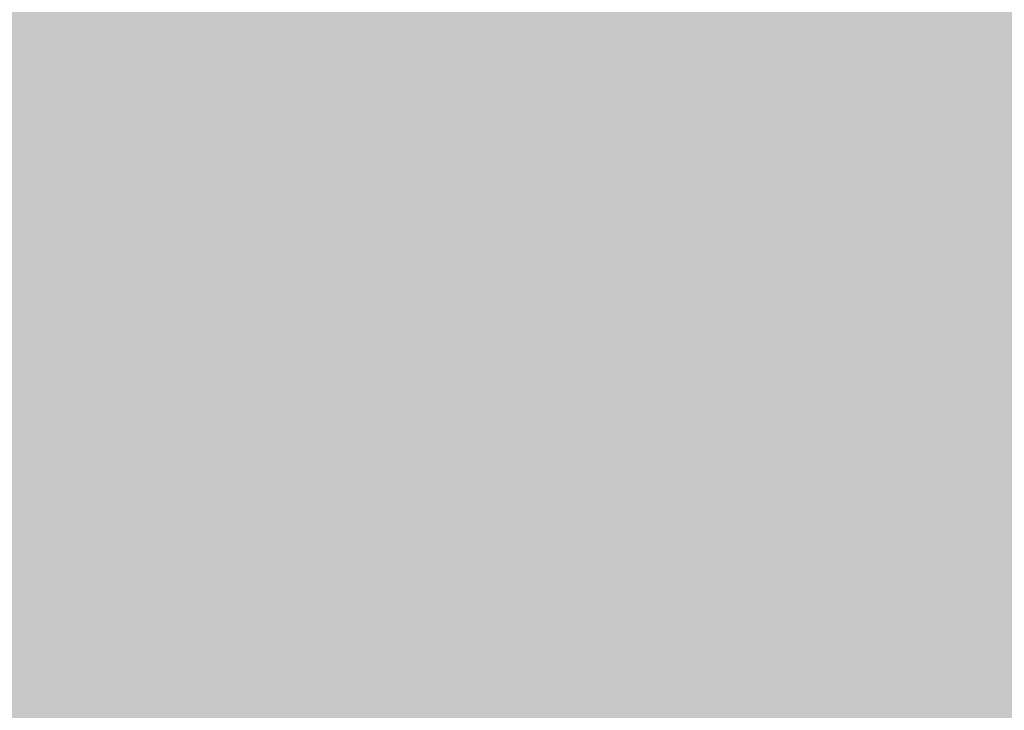
# Model space of a CAD drawing. Units: inches. Extents: x 2091 to 2899, y 967 to 2217.
# Tile 165 of 256: x 2203.144443 to 2203.14684, y 1152.248741 to 1152.250422. Entities that reach past the tile are written whole.
import ezdxf

# ---------------------------------------------------------------- set-up
doc = ezdxf.new("R2010")
doc.units = ezdxf.units.IN
doc.layers.add('A-WALL-PATT', color=141, linetype='Continuous', lineweight=13, true_color=0xadddf7)

msp = doc.modelspace()

# ---------------------------------------------------------------- hatches: boundary and pattern name
at = {"layer": 'A-WALL-PATT'}
h = msp.add_hatch(color=256, dxfattribs=at)
h.dxf.hatch_style = 1
h.paths.add_polyline_path([(2803.1436027, 2050.9190588), (2203.1436027, 2050.9190588), (2203.1436027, 1090.9190588), (2803.1436027, 1090.9190588)])
h.paths.add_polyline_path([(2635.7988501, 1147.5404649), (2674.5240524, 1147.5404649, 0.376086), (2678.5296653, 1152.8802017), (2678.5296653, 1159.5564734, 0.333335), (2674.524319, 1163.561846), (2674.524319, 1163.5618504), (2674.524319, 1192.9343904), (2635.8059707, 1192.9343904), (2597.0876225, 1192.9343904), (2597.0876225, 1163.561846, 0.333335), (2593.0822761, 1159.5564734), (2593.0822761, 1152.8802017, 0.376086), (2597.087889, 1147.5404649)], flags=0)
h.paths.add_polyline_path([(2436.0104329, 1278.2407784, 0.000483), (2435.9526433, 1278.215027, -0.001328), (2435.9356253, 1278.1116934, -0.001711), (2436.1164401, 1278.0407583, 0.002185)], flags=0)
h.paths.add_polyline_path([(2794.1436027, 1143.4190588), (2794.1436027, 1347.4190588), (2543.3701706, 1347.4190588), (2543.3701706, 1351.9190588), (2794.1436027, 1351.9190588), (2794.1436027, 1392.7135549), (2793.9473982, 1392.7135549), (2793.9473982, 1473.5368999), (2794.1436027, 1473.5368999), (2794.1436027, 1531.9190588), (2650.1436027, 1531.9190588), (2650.1436027, 1536.4190588), (2794.1436027, 1536.4190588), (2794.1436027, 1692.4190588), (2609.3756095, 1692.4190588), (2609.3756095, 1644.4190588), (2604.8756095, 1644.4190588), (2604.8756095, 1744.9190588), (2609.3756095, 1744.9190588), (2609.3756095, 1696.9190588), (2794.1436027, 1696.9190588), (2794.1436027, 1780.9190588), (2609.6436027, 1780.9190588), (2493.8756095, 1780.9190588), (2493.8756095, 1785.4190588), (2609.6436027, 1785.4190588), (2794.1436027, 1785.4190588), (2794.1436027, 1847.9388214), (2793.9512217, 1847.9388214), (2793.9512217, 1928.7621663), (2794.1436027, 1928.7621663), (2794.1436027, 1941.4190588), (2614.1436027, 1941.4190588), (2614.1436027, 1821.4190588), (2609.6436027, 1821.4190588), (2609.6436027, 1941.4190588), (2392.1436027, 1941.4190588), (2392.1436027, 1819.9190588), (2387.6436027, 1819.9190588), (2387.6436027, 1941.4190588), (2212.1436027, 1941.4190588), (2212.1436027, 1783.9190588), (2392.1436027, 1783.9190588), (2392.1436027, 1780.9190588), (2212.1436027, 1780.9190588), (2212.1436027, 1629.4190588), (2387.6436027, 1629.4190588), (2387.6436027, 1744.9190588), (2392.1436027, 1744.9190588), (2392.1436027, 1627.9190588), (2317.1436027, 1627.9190588), (2317.1436027, 1551.4190588), (2317.1436027, 1536.4190588), (2459.3835909, 1536.4190588), (2459.3835909, 1602.3964802), (2463.8835909, 1602.3964802), (2463.8835909, 1531.9190588), (2456.6436027, 1531.9190588), (2456.6436027, 1529.9190588), (2452.1436027, 1529.9190588), (2452.1436027, 1531.9190588), (2312.6436027, 1531.9190588), (2312.6436027, 1551.4190588), (2306.1436027, 1551.4190588), (2306.1436027, 1555.9190588), (2308.1436027, 1555.9190588), (2308.1436027, 1551.4190588), (2312.6436027, 1551.4190588), (2312.6436027, 1627.9190588), (2212.1436027, 1627.9190588), (2212.1436027, 1555.9190588), (2270.1436027, 1555.9190588), (2270.1436027, 1551.4190588), (2212.1436027, 1551.4190588), (2212.1436027, 1351.9190588), (2272.1436027, 1351.9190588), (2272.1436027, 1347.4190588), (2212.1436027, 1347.4190588), (2212.1436027, 1275.4190588), (2308.1436027, 1275.4190588), (2308.1436027, 1351.9190588), (2452.1436027, 1351.9190588), (2452.1436027, 1493.9190588), (2456.6436027, 1493.9190588), (2456.6436027, 1347.4190588), (2312.6436027, 1347.4190588), (2312.6436027, 1270.9190588), (2212.1436027, 1270.9190588), (2212.1436027, 1099.9190588), (2281.2375229, 1099.9190588), (2282.8710413, 1110.9138034), (2282.0083413, 1116.9966034), (2278.5577413, 1121.4204034), (2268.2056413, 1128.0562034), (2272.0876413, 1128.0562034), (2273.8129413, 1131.9270034), (2279.4203413, 1134.6919034), (2285.0278413, 1135.2449034), (2287.6158413, 1137.4568034), (2288.0471413, 1138.0098034), (2289.3411413, 1140.7747034), (2291.0665413, 1139.6687034), (2292.3605413, 1135.2449034), (2295.3798413, 1136.9038034), (2296.2425413, 1135.7979034), (2297.1052413, 1133.0330034), (2300.1246413, 1138.0098034), (2303.1439413, 1138.0098034), (2304.4379413, 1135.7979034), (2303.1439413, 1133.5860034), (2306.5946413, 1134.6919034), (2307.8887413, 1133.0330034), (2310.9080413, 1135.2449034), (2313.9274413, 1134.1389034), (2315.6268599, 1132.4271023), (2308.3200413, 1117.5496034), (2290.2038413, 1109.8079034), (2288.9098413, 1103.1721034), (2289.2723086, 1099.9190588), (2434.9182274, 1099.9190588), (2431.5932274, 1124.7880588), (2429.9302274, 1169.5530588), (2430.9271848, 1240.5196942), (2435.6589255, 1238.1861258), (2437.1352274, 1196.5540588), (2438.7982274, 1143.9730588), (2442.6782274, 1111.9980588), (2446.5582274, 1099.9190588), (2794.1436027, 1099.9190588), (2794.1436027, 1138.9190588), (2548.0324471, 1138.9190588), (2548.0324471, 1143.4190588), (2548.0324471, 1148.8190588), (2546.6684571, 1148.0315588), (2528.6856919, 1179.1786218, 0.256256), (2512.0324471, 1148.8190588), (2512.0324471, 1143.4190588), (2512.0324471, 1138.9190588), (2507.5324471, 1138.9190588), (2507.5324471, 1143.4190588), (2507.5324471, 1148.8190588, 0.256256), (2490.8792023, 1179.1786218), (2472.8964371, 1148.0315588), (2471.5324471, 1148.8190588), (2471.5324471, 1143.4190588), (2467.0324471, 1143.4190588), (2467.0324471, 1269.9457858, 0.039061), (2460.9099871, 1273.5800588), (2467.0324471, 1273.5800588), (2467.0324471, 1286.3253638, 0.014511), (2465.2161944, 1286.7619052), (2467.0324471, 1287.0525761), (2467.0324471, 1323.4190588), (2471.5324471, 1323.4190588), (2471.5324471, 1148.8190588), (2489.5324471, 1179.9959734), (2490.8964371, 1179.2084734), (2490.8792023, 1179.1786218, -0.256256), (2507.5324471, 1148.8190588), (2507.5324471, 1143.4190588), (2512.0324471, 1143.4190588), (2512.0324471, 1148.8190588, -0.256256), (2528.6856919, 1179.1786218), (2528.6684571, 1179.2084734), (2530.0324471, 1179.9959734), (2548.0324471, 1148.8190588), (2548.0324471, 1143.4190588)], flags=16)
h.paths.add_polyline_path([(2607.7685461, 1200.9450832), (2607.7685461, 1265.0306251), (2597.0876225, 1281.0520106), (2619.7845852, 1281.0520106), (2627.795278, 1337.1268598), (2635.7988501, 1337.1268598), (2643.8166634, 1337.1268598), (2651.8273562, 1281.0520106), (2674.524319, 1281.0520106), (2663.8433953, 1265.0306251), (2663.8433953, 1200.9450832), (2635.8059707, 1200.9450832)], flags=0)
edge = h.paths.add_edge_path(flags=0)
edge.add_ellipse((13303.8962153, 1272.9987247), major_axis=(-10595.3130399, 0.0000005), ratio=0.842303870086, start_angle=0.62823721906, end_angle=0.64655409989, ccw=False)
edge.add_ellipse((2711.7004495, 1156.8526781), major_axis=(2.2197691, 0), ratio=0.84230387, start_angle=111.5352435, end_angle=180.6282372, ccw=False)
edge.add_ellipse((13303.1562922, 1272.9987246), major_axis=(-10593.0263064, 0), ratio=0.842303869544, start_angle=0.52827147182, end_angle=0.64655409706, ccw=False)
edge.add_line((2710.7645961, 1175.3332951), (2710.1299858, 1175.3332951))
edge.add_ellipse((2710.1299858, 1176.5797752), major_axis=(1.4798461, 0), ratio=0.84230387, start_angle=180, end_angle=270, ccw=False)
edge.add_line((2708.6501397, 1176.5797752), (2708.6501397, 1200.7829144))
edge.add_ellipse((2710.1299858, 1200.7829144), major_axis=(1.4798461, 0), ratio=0.84230387, start_angle=90, end_angle=180, ccw=False)
edge.add_line((2710.1299858, 1202.0293944), (2710.4650752, 1202.0293944))
edge.add_ellipse((13303.1562922, 1272.9987246), major_axis=(-10593.0263064, 0), ratio=0.842303869544, start_angle=-0.09022908859, end_angle=0.38386677879, ccw=False)
edge.add_ellipse((2710.1299858, 1290.9270308), major_axis=(-1.4798461, 0), ratio=0.84230387, start_angle=0, end_angle=90, ccw=False)
edge.add_line((2708.6501397, 1290.9270308), (2708.6501397, 1315.13017))
edge.add_ellipse((2710.1299858, 1315.13017), major_axis=(-1.4798461, 0), ratio=0.84230387, start_angle=-90, end_angle=0, ccw=False)
edge.add_line((2710.1299858, 1316.3766501), (2710.7063141, 1316.3766501))
edge.add_ellipse((3238.4017202, 1296.2895655), major_axis=(528.2339998, 0), ratio=0.84230386954, start_angle=176.349572414, end_angle=177.820049686, ccw=False)
edge.add_ellipse((2775.0630432, 1071.4506962), major_axis=(313.3077613, 0), ratio=0.84230386954, start_angle=102.125965552, end_angle=103.780528989, ccw=False)
edge.add_ellipse((2775.0630432, 1078.3056979), major_axis=(-305.3028915, 0), ratio=0.84230386955, start_angle=-79.790461003, end_angle=-77.555372706, ccw=False)
edge.add_ellipse((2695.1417666, 1541.9753825), major_axis=(-250.9602162, 0), ratio=0.84230386954, start_angle=99.256566007, end_angle=102.554932644)
edge.add_line((2741.4103262, 1334.2142554), (2747.1325454, 1337.3784768))
edge.add_ellipse((2747.5386163, 1336.8574776), major_axis=(-0.739923, 0), ratio=0.84230387, start_angle=270, end_angle=307.9331305, ccw=False)
edge.add_ellipse((2747.5386163, 1336.8574776), major_axis=(-0.739923, 0), ratio=0.84230387, start_angle=232.0668695, end_angle=270, ccw=False)
edge.add_line((2747.9446872, 1337.3784768), (2753.6669064, 1334.2142554))
edge.add_ellipse((2799.935466, 1541.9753825), major_axis=(250.9602162, 0), ratio=0.84230386954, start_angle=257.445067356, end_angle=260.743433993)
edge.add_ellipse((2720.0141894, 1078.3056979), major_axis=(305.3028915, 0), ratio=0.84230386954, start_angle=77.555372707, end_angle=79.790461003, ccw=False)
edge.add_ellipse((2720.0141894, 1071.4506962), major_axis=(-313.3077613, 0), ratio=0.84230386954, start_angle=256.219471011, end_angle=257.874034448, ccw=False)
edge.add_ellipse((2256.6755124, 1296.2895655), major_axis=(-528.2339998, 0), ratio=0.84230386954, start_angle=182.179950314, end_angle=183.650427586, ccw=False)
edge.add_line((2784.3709184, 1316.3766501), (2784.9472468, 1316.3766501))
edge.add_ellipse((2784.9472468, 1315.13017), major_axis=(1.4798461, 0), ratio=0.84230387, start_angle=0, end_angle=90, ccw=False)
edge.add_line((2786.4270928, 1315.13017), (2786.4270928, 1290.9270308))
edge.add_ellipse((2784.9472468, 1290.9270308), major_axis=(1.4798461, 0), ratio=0.84230387, start_angle=270, end_angle=360, ccw=False)
edge.add_ellipse((-7808.0790596, 1272.9987246), major_axis=(10593.0263063, 0), ratio=0.842303869544, start_angle=-0.38386677879, end_angle=0.09022908859, ccw=False)
edge.add_line((2784.6121574, 1202.0293944), (2784.9472468, 1202.0293944))
edge.add_ellipse((2784.9472468, 1200.7829144), major_axis=(1.4798461, 0), ratio=0.84230387, start_angle=0, end_angle=90, ccw=False)
edge.add_line((2786.4270928, 1200.7829144), (2786.4270928, 1176.5797752))
edge.add_ellipse((2784.9472468, 1176.5797752), major_axis=(-1.4798461, 0), ratio=0.84230387, start_angle=90, end_angle=180, ccw=False)
edge.add_line((2784.9472468, 1175.3332951), (2784.3126365, 1175.3332951))
edge.add_ellipse((-7808.0790596, 1272.9987246), major_axis=(10593.0263063, 0), ratio=0.842303869544, start_angle=-0.61864319632, end_angle=-0.52827147182, ccw=False)
edge.add_ellipse((2783.3767831, 1156.8526781), major_axis=(-2.2197691, 0), ratio=0.84230387, start_angle=179.3717628, end_angle=248.4647566, ccw=False)
edge.add_ellipse((-7808.8189826, 1272.9987246), major_axis=(-10595.3130398, 0.0000036), ratio=0.842303865762, start_angle=179.3534459226, end_angle=179.37176280343, ccw=False)
edge.add_ellipse((2780.2973026, 1153.500793), major_axis=(-5.2464256, 0), ratio=0.84230387, start_angle=90, end_angle=179.3534459, ccw=False)
edge.add_line((2780.2973026, 1149.0817084), (2714.77993, 1149.0817084))
edge.add_ellipse((2714.77993, 1153.500793), major_axis=(5.2464256, 0), ratio=0.84230387, start_angle=180.6465541, end_angle=270, ccw=False)
edge = h.paths.add_edge_path(flags=0)
edge.add_line((2718.1873674, 1151.0078329), (2718.1873674, 1170.4723638))
edge.add_ellipse((2721.1470595, 1170.4723638), major_axis=(-2.9596921, 0), ratio=0.84230387, start_angle=-90, end_angle=0, ccw=False)
edge.add_line((2721.1470595, 1172.965324), (2773.9301731, 1172.965324))
edge.add_ellipse((2773.9301731, 1170.4723638), major_axis=(-2.9596921, 0), ratio=0.84230387, start_angle=180, end_angle=270, ccw=False)
edge.add_line((2776.8898652, 1170.4723638), (2776.8898652, 1151.0078329))
edge.add_line((2776.8898652, 1151.0078329), (2718.1873674, 1151.0078329))
edge = h.paths.add_edge_path(flags=0)
edge.add_line((2718.1873674, 1180.2341502), (2718.1873674, 1199.0578342))
edge.add_ellipse((2747.5386163, 1320.3986402), major_axis=(147.0179239, 0), ratio=0.84230386954, start_angle=256.40186531, end_angle=283.59813469)
edge.add_line((2776.8898652, 1199.0578342), (2776.8898652, 1180.2341502))
edge.add_ellipse((2747.5386163, 1301.5749562), major_axis=(147.0179239, 0), ratio=0.84230386954, start_angle=256.40186531, end_angle=283.59813469, ccw=False)
edge = h.paths.add_edge_path(flags=0)
edge.add_ellipse((13303.1562922, 1272.9987246), major_axis=(-10591.5464603, 0), ratio=0.842303869555, start_angle=0.05559431352, end_angle=0.37776419393, ccw=False)
edge.add_line((2711.6168595, 1262.7217103), (2715.6674076, 1249.4953957))
edge.add_ellipse((6413.8919626, 1241.691919), major_axis=(-3698.2361592, 0), ratio=0.842303869547, start_angle=-0.120897369, end_angle=0.3640763489)
edge.add_line((2715.7610383, 1218.1924547), (2711.9343065, 1203.167361))
edge = h.paths.add_edge_path(flags=0)
edge.add_line((2718.1873674, 1251.074566), (2716.0024854, 1267.4504351))
edge.add_ellipse((2742.1511746, 1202.1895399), major_axis=(81.7725845, 0), ratio=0.8423038695, start_angle=94.277420963, end_angle=111.834953797, ccw=False)
edge.add_line((2737.0097482, 1270.9306255), (2758.0674844, 1270.9306255))
edge.add_ellipse((2752.926058, 1202.1895399), major_axis=(81.7725845, 0), ratio=0.8423038695, start_angle=68.165046203, end_angle=85.722579037, ccw=False)
edge.add_line((2779.0747472, 1267.4504351), (2776.8898652, 1251.074566))
edge.add_ellipse((2750.3380588, 1187.8853558), major_axis=(79.5796641, 0), ratio=0.8423038695, start_angle=67.208085122, end_angle=85.129930403)
edge.add_line((2756.0346562, 1254.7436557), (2739.0425764, 1254.7436557))
edge.add_ellipse((2744.7391738, 1187.8853558), major_axis=(79.5796641, 0), ratio=0.8423038695, start_angle=94.870069597, end_angle=112.791914878)
edge = h.paths.add_edge_path(flags=0)
edge.add_line((2783.1429261, 1203.167361), (2779.3161943, 1218.1924547))
edge.add_ellipse((-918.81473, 1241.691919), major_axis=(3698.2361592, 0), ratio=0.842303869546, start_angle=-0.3640763489, end_angle=0.120897369)
edge.add_line((2779.409825, 1249.4953957), (2783.4603731, 1262.7217103))
edge.add_ellipse((-7808.0790596, 1272.9987246), major_axis=(-10591.5464603, 0), ratio=0.84230386954, start_angle=179.6222358061, end_angle=179.94440568651, ccw=False)
edge = h.paths.add_edge_path(flags=0)
edge.add_ellipse((2734.2008921, 1286.6904402), major_axis=(-0.3566086, 6.3400775), ratio=0.603833576, start_angle=89.00201428, end_angle=253.65740805, ccw=False)
edge.add_line((2730.3690013, 1286.5418057), (2730.3690013, 1301.3519803))
edge.add_line((2730.3690013, 1301.3519803), (2735.9133107, 1305.2148028))
edge.add_ellipse((2736.3849168, 1304.7345612), major_axis=(0.739923, 0), ratio=0.84230387, start_angle=90, end_angle=134.4802109, ccw=False)
edge.add_line((2736.3849168, 1305.3578013), (2738.0327829, 1305.3578013))
edge.add_line((2738.0327829, 1305.3578013), (2738.0327829, 1307.7079274))
edge.add_ellipse((2794.201642, 1307.7079274), major_axis=(56.168859, 0), ratio=0.8423038695, start_angle=150.5614304, end_angle=180, ccw=False)
edge.add_ellipse((2700.8755906, 1307.7079274), major_axis=(-56.168859, 0), ratio=0.8423038695, start_angle=180, end_angle=209.4385696, ccw=False)
edge.add_line((2757.0444497, 1307.7079274), (2757.0444497, 1305.3578013))
edge.add_line((2757.0444497, 1305.3578013), (2758.6923157, 1305.3578013))
edge.add_ellipse((2758.6923157, 1304.7345612), major_axis=(-0.739923, 0), ratio=0.84230387, start_angle=225.5197891, end_angle=270, ccw=False)
edge.add_line((2759.1639219, 1305.2148028), (2764.7082312, 1301.3519803))
edge.add_line((2764.7082312, 1301.3519803), (2764.7082312, 1286.5418057))
edge.add_ellipse((2760.8763405, 1286.6904402), major_axis=(0.3566086, 6.3400775), ratio=0.603833576, start_angle=106.34259195, end_angle=270.99798572, ccw=False)
edge.add_line((2757.0444497, 1285.7970896), (2757.0444497, 1307.7079274))
edge.add_ellipse((2700.8755906, 1307.7079274), major_axis=(-56.168859, 0), ratio=0.8423038695, start_angle=180, end_angle=209.4385696)
edge.add_ellipse((2794.201642, 1307.7079274), major_axis=(56.168859, 0), ratio=0.8423038695, start_angle=150.5614304, end_angle=180)
edge.add_line((2738.0327829, 1307.7079274), (2738.0327829, 1285.7970896))
h.paths.add_polyline_path([(2417.8122727, 1104.449704), (2413.4922727, 1102.529704), (2410.6122727, 1103.969704), (2409.1722727, 1106.369704), (2407.2522727, 1107.329704), (2406.2922727, 1109.729704), (2405.3322727, 1114.049704), (2405.3322727, 1117.889704), (2406.2922727, 1120.129704), (2407.2522727, 1119.809704), (2408.8483218, 1118.3276585), (2410.1739451, 1119.4241703), (2410.2112727, 1120.405704), (2411.0407305, 1121.4190541), (2410.6992727, 1119.858704), (2410.1739451, 1119.4241703), (2410.0884515, 1117.1761095), (2411.1328361, 1116.2063237), (2413.9722727, 1119.329704), (2416.8522727, 1120.769704), (2416.8697209, 1120.7987842), (2417.0350713, 1119.4051162), (2417.8962134, 1118.1433844), (2418.2922727, 1118.369704), (2419.5444467, 1120.0392692), (2419.3609153, 1118.387487), (2419.0321078, 1119.3561507), (2418.3989394, 1118.5119262), (2419.2522727, 1114.529704), (2418.7940909, 1107.1987949)], flags=0)
h.paths.add_polyline_path([(2508.8701706, 1347.4190588), (2508.3701706, 1347.4190588), (2508.3701706, 1351.9190588), (2508.8701706, 1351.9190588)], flags=0)
h.paths.add_polyline_path([(2473.3701706, 1347.4190588), (2472.3701706, 1347.4190588), (2467.8701706, 1347.4190588), (2467.8701706, 1455.4190588), (2472.3701706, 1455.4190588), (2472.3701706, 1352.4190588), (2473.3701706, 1352.4190588)], flags=0)
h.paths.add_polyline_path([(2352.106244, 1217.4461971), (2349.226244, 1218.8861971), (2347.786244, 1221.2861971), (2345.866244, 1222.2461971), (2344.906244, 1224.6461971), (2343.946244, 1228.9661971), (2343.946244, 1232.8061971), (2344.906244, 1235.0461971), (2345.866244, 1234.7261971), (2347.4622931, 1233.2441515), (2348.7879164, 1234.3406634), (2348.825244, 1235.3221971), (2349.6547018, 1236.3355471), (2349.313244, 1234.7751971), (2348.7879164, 1234.3406634), (2348.7024228, 1232.0926025), (2349.7468074, 1231.1228168), (2352.586244, 1234.2461971), (2355.466244, 1235.6861971), (2355.4836921, 1235.7152773), (2355.6490426, 1234.3216093), (2356.5101846, 1233.0598774), (2356.906244, 1233.2861971), (2358.1584179, 1234.9557623), (2357.9748866, 1233.3039801), (2357.6460791, 1234.2726438), (2357.0129107, 1233.4284193), (2357.866244, 1229.4461971), (2357.4080622, 1222.115288), (2356.426244, 1219.3661971)], flags=0)
h.paths.add_polyline_path([(2348.2967999, 1112.2244204), (2347.0137999, 1112.3104204), (2345.5297999, 1114.1274204), (2345.7317999, 1115.8584204), (2346.8117999, 1116.9824204), (2346.8117999, 1114.6464204), (2345.8667999, 1114.2144204), (2346.8797999, 1114.3004204)], flags=0)
h.paths.add_polyline_path([(2347.0137999, 1110.9264204), (2346.2717999, 1110.4934204), (2346.6097999, 1111.1864204)], flags=0)
h.paths.add_polyline_path([(2345.8667999, 1118.1944204), (2345.5297999, 1117.3294204), (2343.7077999, 1118.0214204), (2344.3827999, 1118.6264204)], flags=0)
h.paths.add_polyline_path([(2346.6767999, 1109.2824204), (2346.0697999, 1108.0714204), (2345.8667999, 1110.0614204)], flags=0)
h.paths.add_polyline_path([(2345.0567999, 1119.7514204), (2343.6397999, 1119.7514204), (2343.9777999, 1121.1354204)], flags=0)
h.paths.add_polyline_path([(2345.2597999, 1116.5504204), (2345.1247999, 1115.8584204), (2344.9217999, 1115.6854204), (2344.7197999, 1116.3774204)], flags=0)
h.paths.add_polyline_path([(2345.6647999, 1112.3104204), (2345.4617999, 1111.5324204), (2344.0447999, 1111.9644204), (2344.6517999, 1112.5704204)], flags=0)
h.paths.add_polyline_path([(2345.1917999, 1113.3494204), (2344.4497999, 1113.8684204), (2344.7197999, 1114.3874204)], flags=0)
h.paths.add_polyline_path([(2344.6517999, 1116.8094204), (2344.1797999, 1115.6854204), (2344.6517999, 1115.3394204), (2343.9097999, 1114.9064204), (2343.0327999, 1115.9444204), (2343.6397999, 1116.4634204)], flags=0)
h.paths.add_polyline_path([(2345.8667999, 1106.6864204), (2344.9897999, 1105.5624204), (2344.5167999, 1106.6004204)], flags=0)
h.paths.add_polyline_path([(2344.8547999, 1110.0614204), (2344.5167999, 1109.2824204), (2344.1127999, 1109.7154204)], flags=0)
h.paths.add_polyline_path([(2344.0447999, 1113.5224204), (2343.4377999, 1113.0894204), (2342.7627999, 1113.9544204)], flags=0)
h.paths.add_polyline_path([(2344.3147999, 1111.0124204), (2342.9647999, 1110.3204204), (2342.9647999, 1111.0994204)], flags=0)
h.paths.add_polyline_path([(2345.1247999, 1104.6974204), (2344.5847999, 1103.7454204), (2344.4497999, 1104.2644204)], flags=0)
h.paths.add_polyline_path([(2342.8297999, 1121.2224204), (2341.7497999, 1120.5304204), (2340.5357999, 1121.0494204), (2340.1307999, 1121.8284204), (2340.6707999, 1122.9524204), (2341.1427999, 1121.8284204), (2341.6147999, 1122.0014204)], flags=0)
h.paths.add_polyline_path([(2342.9647999, 1119.7514204), (2343.0327999, 1118.4534204), (2342.0877999, 1118.0214204), (2342.0197999, 1119.4914204)], flags=0)
h.paths.add_polyline_path([(2342.6947999, 1116.8964204), (2341.9527999, 1116.6364204), (2342.0197999, 1117.3294204)], flags=0)
h.paths.add_polyline_path([(2343.0327999, 1112.2244204), (2342.0197999, 1111.7914204), (2341.5477999, 1112.2244204), (2342.3577999, 1113.3494204)], flags=0)
h.paths.add_polyline_path([(2343.7747999, 1104.4374204), (2342.6277999, 1102.8804204), (2342.6947999, 1104.6104204), (2343.4377999, 1105.1294204)], flags=0)
h.paths.add_polyline_path([(2342.0197999, 1115.0794204), (2340.8057999, 1115.5124204), (2340.9407999, 1116.3774204)], flags=0)
h.paths.add_polyline_path([(2341.4807999, 1120.0974204), (2341.4807999, 1119.4054204), (2341.0757999, 1119.5784204), (2341.1427999, 1120.0974204)], flags=0)
h.paths.add_polyline_path([(2341.8177999, 1114.4734204), (2340.9407999, 1113.0894204), (2340.8057999, 1114.5604204)], flags=0)
h.paths.add_polyline_path([(2341.1427999, 1118.5404204), (2340.9407999, 1116.9824204), (2339.0507999, 1117.6754204), (2339.0507999, 1118.6264204)], flags=0)
h.paths.add_polyline_path([(2342.6947999, 1101.6684204), (2341.9527999, 1101.8414204), (2342.5597999, 1102.3614204)], flags=0)
h.paths.add_polyline_path([(2340.3327999, 1119.6654204), (2338.4437999, 1119.5784204), (2337.9037999, 1120.3574204), (2339.6577999, 1120.6164204)], flags=0)
h.paths.add_polyline_path([(2340.3327999, 1115.3394204), (2340.0627999, 1113.6954204), (2339.3877999, 1115.3394204)], flags=0)
h.paths.add_polyline_path([(2341.8177999, 1103.8314204), (2341.5477999, 1102.8804204), (2341.1427999, 1103.6584204)], flags=0)
h.paths.add_polyline_path([(2339.0507999, 1122.8664204), (2337.2957999, 1121.8284204), (2337.0937999, 1123.1254204), (2337.7687999, 1123.8184204)], flags=0)
h.paths.add_polyline_path([(2339.1177999, 1121.7414204), (2338.8477999, 1121.2224204), (2338.1737999, 1121.0494204), (2338.3757999, 1121.5684204)], flags=0)
h.paths.add_polyline_path([(2339.1857999, 1119.3194204), (2338.6457999, 1118.7134204), (2338.2407999, 1118.1074204), (2338.2407999, 1118.8864204)], flags=0)
h.paths.add_polyline_path([(2341.1427999, 1101.9284204), (2340.6027999, 1101.2364204), (2340.0627999, 1101.8414204), (2340.6027999, 1102.3614204)], flags=0)
h.paths.add_polyline_path([(2337.6337999, 1117.7614204), (2336.6207999, 1118.2804204), (2337.2957999, 1118.9724204)], flags=0)
h.paths.add_polyline_path([(2336.8237999, 1119.5784204), (2334.7987999, 1118.9724204), (2335.2037999, 1120.3574204), (2336.5537999, 1120.8764204)], flags=0)
h.paths.add_polyline_path([(2339.1177999, 1100.4574204), (2337.3637999, 1100.5434204), (2336.7557999, 1101.2364204)], flags=0)
h.paths.add_polyline_path([(2336.3507999, 1122.4334204), (2336.0137999, 1121.9144204), (2334.9337999, 1122.4334204), (2334.5287999, 1123.4714204), (2335.7437999, 1122.7794204)], flags=0)
h.paths.add_polyline_path([(2334.7317999, 1120.8764204), (2334.2587999, 1120.3574204), (2334.0567999, 1120.7894204), (2334.5967999, 1121.3084204)], flags=0)
h.paths.add_polyline_path([(2334.4617999, 1122.1744204), (2332.5717999, 1121.3084204), (2331.3567999, 1122.1744204), (2332.0997999, 1122.8664204)], flags=0)
h.paths.add_polyline_path([(2334.2587999, 1118.5404204), (2333.3817999, 1118.4534204), (2333.6517999, 1119.3194204)], flags=0)
h.paths.add_polyline_path([(2335.5417999, 1102.2744204), (2334.1917999, 1102.6204204), (2335.2717999, 1103.3124204)], flags=0)
h.paths.add_polyline_path([(2332.7067999, 1119.6654204), (2331.6947999, 1120.4434204), (2332.5047999, 1120.7894204)], flags=0)
h.paths.add_polyline_path([(2334.7317999, 1101.1494204), (2333.5167999, 1101.5824204), (2333.9887999, 1101.7554204)], flags=0)
h.paths.add_polyline_path([(2332.6397999, 1116.6364204), (2331.0867999, 1116.2904204), (2331.9647999, 1118.1944204)], flags=0)
h.paths.add_polyline_path([(2330.7497999, 1121.5684204), (2330.2767999, 1120.2704204), (2328.5227999, 1119.3194204), (2328.9947999, 1121.0494204)], flags=0)
h.paths.add_polyline_path([(2330.7497999, 1118.6264204), (2330.0077999, 1117.5024204), (2329.8727999, 1118.0214204)], flags=0)
h.paths.add_polyline_path([(2332.0997999, 1102.3614204), (2330.5467999, 1102.0144204), (2331.6947999, 1102.9664204)], flags=0)
h.paths.add_polyline_path([(2329.5347999, 1113.6084204), (2329.0627999, 1112.3104204), (2328.5897999, 1113.3494204)], flags=0)
h.paths.add_polyline_path([(2328.3877999, 1117.8484204), (2327.5097999, 1116.5504204), (2327.1727999, 1117.7614204)], flags=0)
h.paths.add_polyline_path([(2329.7377999, 1106.5134204), (2329.5347999, 1105.3024204), (2328.2527999, 1106.0814204)], flags=0)
h.paths.add_polyline_path([(2328.6577999, 1114.3874204), (2328.0497999, 1114.1274204), (2328.3197999, 1114.9064204)], flags=0)
h.paths.add_polyline_path([(2328.3197999, 1112.2244204), (2327.1057999, 1112.1374204), (2326.7007999, 1112.6564204)], flags=0)
h.paths.add_polyline_path([(2326.9027999, 1115.2524204), (2326.7007999, 1114.1274204), (2325.2157999, 1113.6084204), (2326.0927999, 1115.3394204)], flags=0)
h.paths.add_polyline_path([(2326.6327999, 1108.3304204), (2326.0927999, 1107.3794204), (2325.8907999, 1108.5034204), (2326.4977999, 1109.1094204)], flags=0)
h.paths.add_polyline_path([(2615.1436027, 1531.9190588), (2609.6436027, 1531.9190588), (2609.6436027, 1620.4190588), (2614.1436027, 1620.4190588), (2614.1436027, 1536.4190588), (2615.1436027, 1536.4190588)], flags=0)
h.paths.add_polyline_path([(2545.1436027, 1563.4190588), (2464.1436027, 1563.4190588), (2464.1436027, 1632.4190588), (2509.1436027, 1632.4190588), (2509.1436027, 1627.9190588), (2509.1436027, 1603.9190588), (2468.6436027, 1603.9190588), (2468.6436027, 1567.9190588), (2540.6436027, 1567.9190588), (2540.6436027, 1591.9190588), (2545.1436027, 1591.9190588)], flags=0)
h.paths.add_polyline_path([(2388.9690483, 1549.985735), (2357.4341811, 1549.985735), (2357.4341811, 1623.3607783), (2399.3627772, 1623.3607783), (2435.6894654, 1623.3607783), (2435.5925469, 1602.5592734), (2435.5925469, 1602.3964802), (2388.9690483, 1602.3964802)], flags=0)
h.paths.add_polyline_path([(2388.8806282, 1555.8091511), (2374.9044295, 1555.8091511), (2374.9044295, 1600.5715641), (2374.9044295, 1615.4576454), (2406.3508766, 1615.4576454), (2406.3508766, 1618.9394309), (2412.1742927, 1615.4576454), (2406.3508766, 1611.9758599), (2406.3508766, 1615.4576454), (2388.8806282, 1615.4576454)], flags=0)
h.paths.add_polyline_path([(2568.8756095, 1644.4190588), (2453.3756095, 1644.4190588), (2453.3756095, 1785.4190588), (2457.8756095, 1785.4190588), (2457.8756095, 1648.9190588), (2568.8756095, 1648.9190588)], flags=0)
h.paths.add_polyline_path([(2212.1436027, 1945.9190588), (2212.1436027, 2041.9190588), (2794.1436027, 2041.9190588), (2794.1436027, 1945.9190588)], flags=16)
h.paths.add_polyline_path([(2271.0827276, 1964.3172377), (2776.852968, 1964.3172377), (2776.852968, 2037.1696226), (2271.0827276, 2037.1696226)], flags=8)
h.paths.add_polyline_path([(2380.6492852, 1536.8241435), (2461.0408087, 1536.8241435), (2461.0408087, 1554.6525871), (2380.6492852, 1554.6525871)], flags=8)
h.paths.add_polyline_path([(2240.7557092, 1609.7254508), (2309.1858294, 1609.7254508), (2309.1858294, 1617.6982037), (2240.7557092, 1617.6982037)], flags=8)
h.paths.add_polyline_path([(2212.6772554, 1313.5041021), (2282.5915203, 1313.5041021), (2282.5915203, 1322.7452389), (2212.6772554, 1322.7452389)], flags=8)
h.paths.add_polyline_path([(2457.111976, 1114.778574), (2558.4815807, 1114.778574), (2558.4815807, 1142.2196823), (2457.111976, 1142.2196823)], flags=8)
h.paths.add_polyline_path([(2473.4423372, 1273.0100672), (2604.6412257, 1273.0100672), (2604.6412257, 1318.3469349), (2473.4423372, 1318.3469349)], flags=8)
h.paths.add_polyline_path([(2638.8763024, 1626.9774316), (2684.2503675, 1627.9767377), (2684.0384825, 1637.5974944), (2638.6644174, 1636.5981884)], flags=8)
h.paths.add_polyline_path([(2537.5905538, 1453.7934466), (2628.3895472, 1453.7934466), (2628.3895472, 1475.3448114), (2537.5905538, 1475.3448114)], flags=8)
h.paths.add_polyline_path([(2504.1376376, 1714.6323972), (2554.6471875, 1714.6323972), (2554.6471875, 1730.2377115), (2504.1376376, 1730.2377115)], flags=8)
h.paths.add_polyline_path([(2487.5011806, 1575.6518716), (2535.0971214, 1575.6518716), (2535.0971214, 1598.3776456), (2487.5011806, 1598.3776456)], flags=8)
h.paths.add_polyline_path([(2709.0994004, 1735.7102784), (2740.0166009, 1735.7102784), (2740.0166009, 1749.9376406), (2709.0994004, 1749.9376406)], flags=8)
h.paths.add_polyline_path([(2442.4384239, 1792.1716575), (2564.7288353, 1792.1716575), (2564.7288353, 1842.0001626), (2442.4384239, 1842.0001626)], flags=8)
h.paths.add_polyline_path([(2655.8158012, 1809.6440763), (2789.5201425, 1806.6937963), (2790.0849768, 1832.2916379), (2656.3806355, 1835.2419179)], flags=8)
h.paths.add_polyline_path([(2234.8426972, 1797.7201432), (2368.5928512, 1794.7688523), (2369.1607182, 1820.504132), (2235.4105642, 1823.4554229)], flags=8)
h.paths.add_polyline_path([(2245.1384659, 1644.0063348), (2398.4277329, 1640.6238997), (2398.9948417, 1666.3248199), (2245.7055747, 1669.7072549)], flags=8)
h.paths.add_polyline_path([(2306.1428474, 1431.1685186), (2413.7683138, 1428.7936873), (2414.3331481, 1454.3915289), (2306.7076817, 1456.7663602)], flags=8)
h.paths.add_polyline_path([(2306.834582, 1458.2331447), (2393.3804836, 1456.3234487), (2393.9328082, 1481.3543583), (2307.3869066, 1483.2640542)], flags=8)

doc.saveas('drawing.dxf')
